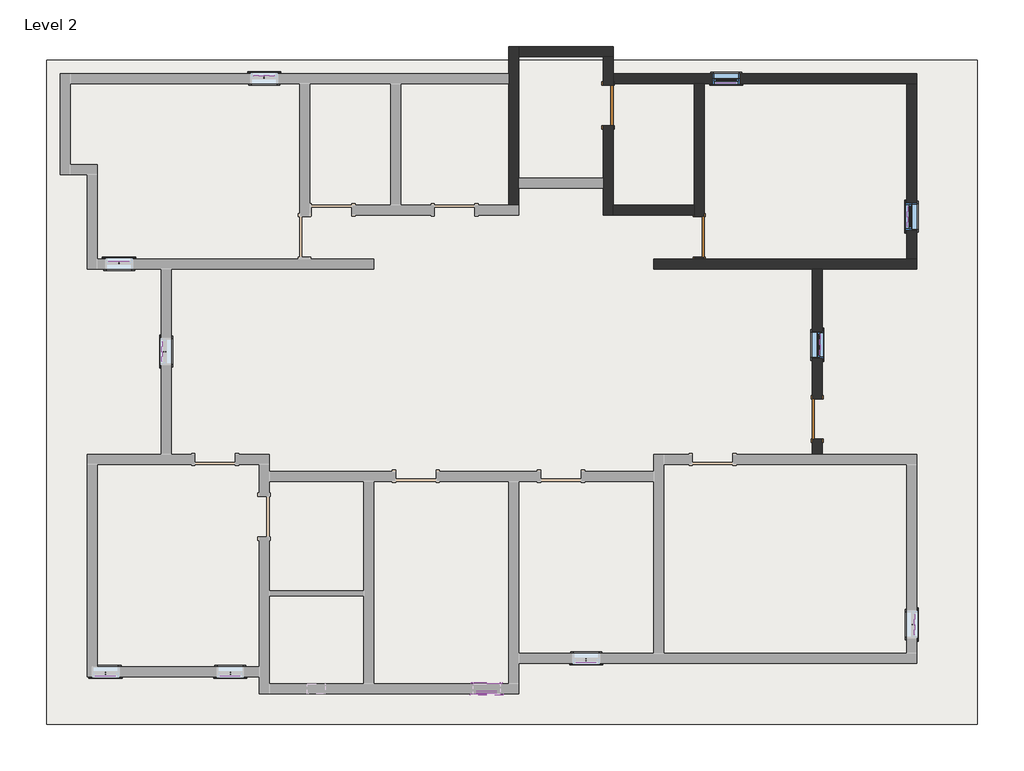
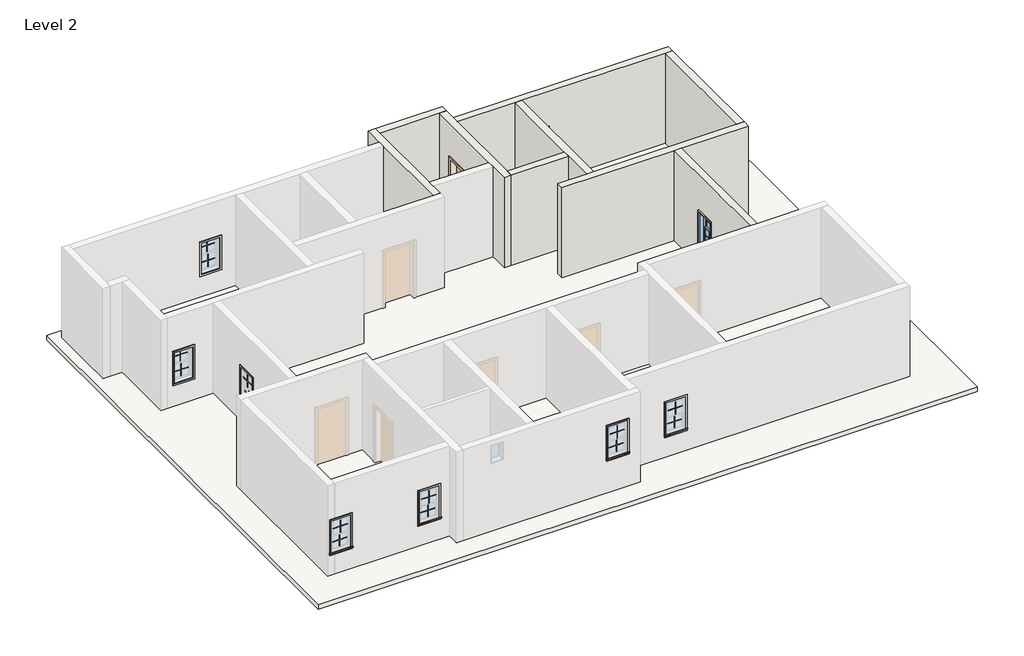
# One storey, part 2 of 2: 44 proxies, 9 walls, 3 doors, 3 windows, 1 roof.
"""IFC4 building model written with IfcOpenShell, lengths in millimetres."""

from ifc_helpers import new_model, si_unit, frame, origin, place, context, project, spatial, polyline, outline, extrude, faceted_brep, transform, mapped, element, save
from components import muntin_pattern_2x2_muntin_pattern_2x2_eba6c5fb, trim_window_exterior_flat_with_sill_278e6a94, trim_window_interior_flat_picture_frame_e9fd5f45, door_89fc3733, door_ef0d591a, window_d92165b9

model = new_model("IFC4")

# Units and contexts
model_context = context("Model", 3, world=origin())
ifc_project = project(units=[si_unit("LENGTHUNIT", "METRE", prefix="MILLI")], contexts=[model_context])

# Site, building, storey
site = spatial("IfcSite", under=ifc_project)
building = spatial("IfcBuilding", under=site)
storey = spatial("IfcBuildingStorey", under=building, Name="Level 2", Elevation=3200.4)

# Proxies
placement = place(None, origin())
muntin_pattern_2x2_muntin_pattern_2x2_shape = muntin_pattern_2x2_muntin_pattern_2x2_eba6c5fb(model_context)
element("IfcBuildingElementProxy", 1, Name="Muntin Pattern_2x2 : Muntin Pattern_2x2", ObjectType="Muntin Pattern_2x2 : Muntin Pattern_2x2", at=placement, inside=storey, context=model_context, shape_type="MappedRepresentation", body=[
    mapped(muntin_pattern_2x2_muntin_pattern_2x2_shape, transform((-9484.8415084, 7932.7685985, 4670.425), x_axis=(1.0, 0.0, 0.0), y_axis=(0.0, 1.0, 0.0), z_axis=(0.0, 0.0, 1.0))),
])
element("IfcBuildingElementProxy", 2, Name="Muntin Pattern_2x2 : Muntin Pattern_2x2", ObjectType="Muntin Pattern_2x2 : Muntin Pattern_2x2", at=placement, inside=storey, context=model_context, shape_type="MappedRepresentation", body=[
    mapped(muntin_pattern_2x2_muntin_pattern_2x2_shape, transform((-9484.8415084, 7888.3185985, 4191.0), x_axis=(1.0, 0.0, 0.0), y_axis=(0.0, 1.0, 0.0), z_axis=(0.0, 0.0, 1.0))),
])
element("IfcBuildingElementProxy", 3, Name="Muntin Pattern_2x2 : Muntin Pattern_2x2", ObjectType="Muntin Pattern_2x2 : Muntin Pattern_2x2", at=placement, inside=storey, context=model_context, shape_type="MappedRepresentation", body=[
    mapped(muntin_pattern_2x2_muntin_pattern_2x2_shape, transform((-12761.4415084, 3741.7685985, 4670.425), x_axis=(1.0, 0.0, 0.0), y_axis=(0.0, 1.0, 0.0), z_axis=(0.0, 0.0, 1.0))),
])
element("IfcBuildingElementProxy", 4, Name="Muntin Pattern_2x2 : Muntin Pattern_2x2", ObjectType="Muntin Pattern_2x2 : Muntin Pattern_2x2", at=placement, inside=storey, context=model_context, shape_type="MappedRepresentation", body=[
    mapped(muntin_pattern_2x2_muntin_pattern_2x2_shape, transform((-12761.4415084, 3697.3185985, 4191.0), x_axis=(1.0, 0.0, 0.0), y_axis=(0.0, 1.0, 0.0), z_axis=(0.0, 0.0, 1.0))),
])
element("IfcBuildingElementProxy", 5, Name="Muntin Pattern_2x2 : Muntin Pattern_2x2", ObjectType="Muntin Pattern_2x2 : Muntin Pattern_2x2", at=placement, inside=storey, context=model_context, shape_type="MappedRepresentation", body=[
    mapped(muntin_pattern_2x2_muntin_pattern_2x2_shape, transform((-13066.2415084, -5637.1814015, 4670.425), x_axis=(-1.0, 0.0, 0.0), y_axis=(0.0, -1.0, 0.0), z_axis=(0.0, 0.0, 1.0))),
])
element("IfcBuildingElementProxy", 6, Name="Muntin Pattern_2x2 : Muntin Pattern_2x2", ObjectType="Muntin Pattern_2x2 : Muntin Pattern_2x2", at=placement, inside=storey, context=model_context, shape_type="MappedRepresentation", body=[
    mapped(muntin_pattern_2x2_muntin_pattern_2x2_shape, transform((-13066.2415084, -5592.7314015, 4191.0), x_axis=(-1.0, 0.0, 0.0), y_axis=(0.0, -1.0, 0.0), z_axis=(0.0, 0.0, 1.0))),
])
element("IfcBuildingElementProxy", 7, Name="Muntin Pattern_2x2 : Muntin Pattern_2x2", ObjectType="Muntin Pattern_2x2 : Muntin Pattern_2x2", at=placement, inside=storey, context=model_context, shape_type="MappedRepresentation", body=[
    mapped(muntin_pattern_2x2_muntin_pattern_2x2_shape, transform((-10246.8415084, -5637.1814015, 4670.425), x_axis=(-1.0, 0.0, 0.0), y_axis=(0.0, -1.0, 0.0), z_axis=(0.0, 0.0, 1.0))),
])
element("IfcBuildingElementProxy", 8, Name="Muntin Pattern_2x2 : Muntin Pattern_2x2", ObjectType="Muntin Pattern_2x2 : Muntin Pattern_2x2", at=placement, inside=storey, context=model_context, shape_type="MappedRepresentation", body=[
    mapped(muntin_pattern_2x2_muntin_pattern_2x2_shape, transform((-10246.8415084, -5592.7314015, 4191.0), x_axis=(-1.0, 0.0, 0.0), y_axis=(0.0, -1.0, 0.0), z_axis=(0.0, 0.0, 1.0))),
])
element("IfcBuildingElementProxy", 9, Name="Muntin Pattern_2x2 : Muntin Pattern_2x2", ObjectType="Muntin Pattern_2x2 : Muntin Pattern_2x2", at=placement, inside=storey, context=model_context, shape_type="MappedRepresentation", body=[
    mapped(muntin_pattern_2x2_muntin_pattern_2x2_shape, transform((954.5584916, 7774.0185985, 4670.425), x_axis=(-1.0, 0.0, 0.0), y_axis=(0.0, -1.0, 0.0), z_axis=(0.0, 0.0, 1.0))),
])
element("IfcBuildingElementProxy", 10, Name="Muntin Pattern_2x2 : Muntin Pattern_2x2", ObjectType="Muntin Pattern_2x2 : Muntin Pattern_2x2", at=placement, inside=storey, context=model_context, shape_type="MappedRepresentation", body=[
    mapped(muntin_pattern_2x2_muntin_pattern_2x2_shape, transform((954.5584916, 7818.4685985, 4191.0), x_axis=(-1.0, 0.0, 0.0), y_axis=(0.0, -1.0, 0.0), z_axis=(0.0, 0.0, 1.0))),
])
element("IfcBuildingElementProxy", 11, Name="Muntin Pattern_2x2 : Muntin Pattern_2x2", ObjectType="Muntin Pattern_2x2 : Muntin Pattern_2x2", at=placement, inside=storey, context=model_context, shape_type="MappedRepresentation", body=[
    mapped(muntin_pattern_2x2_muntin_pattern_2x2_shape, transform((-11774.0165084, 1681.1935985, 4670.425), x_axis=(0.0, 1.0, 0.0), y_axis=(-1.0, 0.0, 0.0), z_axis=(0.0, 0.0, 1.0))),
])
element("IfcBuildingElementProxy", 12, Name="Muntin Pattern_2x2 : Muntin Pattern_2x2", ObjectType="Muntin Pattern_2x2 : Muntin Pattern_2x2", at=placement, inside=storey, context=model_context, shape_type="MappedRepresentation", body=[
    mapped(muntin_pattern_2x2_muntin_pattern_2x2_shape, transform((-11729.5665084, 1681.1935985, 4191.0), x_axis=(0.0, 1.0, 0.0), y_axis=(-1.0, 0.0, 0.0), z_axis=(0.0, 0.0, 1.0))),
])
element("IfcBuildingElementProxy", 13, Name="Muntin Pattern_2x2 : Muntin Pattern_2x2", ObjectType="Muntin Pattern_2x2 : Muntin Pattern_2x2", at=placement, inside=storey, context=model_context, shape_type="MappedRepresentation", body=[
    mapped(muntin_pattern_2x2_muntin_pattern_2x2_shape, transform((-2207.7415084, -5332.3814015, 4670.425), x_axis=(-1.0, 0.0, 0.0), y_axis=(0.0, -1.0, 0.0), z_axis=(0.0, 0.0, 1.0))),
])
element("IfcBuildingElementProxy", 14, Name="Muntin Pattern_2x2 : Muntin Pattern_2x2", ObjectType="Muntin Pattern_2x2 : Muntin Pattern_2x2", at=placement, inside=storey, context=model_context, shape_type="MappedRepresentation", body=[
    mapped(muntin_pattern_2x2_muntin_pattern_2x2_shape, transform((-2207.7415084, -5287.9314015, 4191.0), x_axis=(-1.0, 0.0, 0.0), y_axis=(0.0, -1.0, 0.0), z_axis=(0.0, 0.0, 1.0))),
])
element("IfcBuildingElementProxy", 15, Name="Muntin Pattern_2x2 : Muntin Pattern_2x2", ObjectType="Muntin Pattern_2x2 : Muntin Pattern_2x2", at=placement, inside=storey, context=model_context, shape_type="MappedRepresentation", body=[
    mapped(muntin_pattern_2x2_muntin_pattern_2x2_shape, transform((5224.9334916, -4491.0064015, 4670.425), x_axis=(0.0, -1.0, 0.0), y_axis=(1.0, 0.0, 0.0), z_axis=(0.0, 0.0, 1.0))),
])
element("IfcBuildingElementProxy", 16, Name="Muntin Pattern_2x2 : Muntin Pattern_2x2", ObjectType="Muntin Pattern_2x2 : Muntin Pattern_2x2", at=placement, inside=storey, context=model_context, shape_type="MappedRepresentation", body=[
    mapped(muntin_pattern_2x2_muntin_pattern_2x2_shape, transform((5180.4834916, -4491.0064015, 4191.0), x_axis=(0.0, -1.0, 0.0), y_axis=(1.0, 0.0, 0.0), z_axis=(0.0, 0.0, 1.0))),
])
element("IfcBuildingElementProxy", 17, Name="Muntin Pattern_2x2 : Muntin Pattern_2x2", ObjectType="Muntin Pattern_2x2 : Muntin Pattern_2x2", at=placement, inside=storey, context=model_context, shape_type="MappedRepresentation", body=[
    mapped(muntin_pattern_2x2_muntin_pattern_2x2_shape, transform((3091.3334916, 1833.5935985, 4670.425), x_axis=(0.0, -1.0, 0.0), y_axis=(1.0, 0.0, 0.0), z_axis=(0.0, 0.0, 1.0))),
])
element("IfcBuildingElementProxy", 18, Name="Muntin Pattern_2x2 : Muntin Pattern_2x2", ObjectType="Muntin Pattern_2x2 : Muntin Pattern_2x2", at=placement, inside=storey, context=model_context, shape_type="MappedRepresentation", body=[
    mapped(muntin_pattern_2x2_muntin_pattern_2x2_shape, transform((3046.8834916, 1833.5935985, 4191.0), x_axis=(0.0, -1.0, 0.0), y_axis=(1.0, 0.0, 0.0), z_axis=(0.0, 0.0, 1.0))),
])
element("IfcBuildingElementProxy", 19, Name="Muntin Pattern_2x2 : Muntin Pattern_2x2", ObjectType="Muntin Pattern_2x2 : Muntin Pattern_2x2", at=placement, inside=storey, context=model_context, shape_type="MappedRepresentation", body=[
    mapped(muntin_pattern_2x2_muntin_pattern_2x2_shape, transform((5066.1834916, 4729.1935985, 4670.425), x_axis=(0.0, 1.0, 0.0), y_axis=(-1.0, 0.0, 0.0), z_axis=(0.0, 0.0, 1.0))),
])
element("IfcBuildingElementProxy", 20, Name="Muntin Pattern_2x2 : Muntin Pattern_2x2", ObjectType="Muntin Pattern_2x2 : Muntin Pattern_2x2", at=placement, inside=storey, context=model_context, shape_type="MappedRepresentation", body=[
    mapped(muntin_pattern_2x2_muntin_pattern_2x2_shape, transform((5110.6334916, 4729.1935985, 4191.0), x_axis=(0.0, 1.0, 0.0), y_axis=(-1.0, 0.0, 0.0), z_axis=(0.0, 0.0, 1.0))),
])
element("IfcBuildingElementProxy", 21, Name="Muntin Pattern_2x2 : Muntin Pattern_2x2", ObjectType="Muntin Pattern_2x2 : Muntin Pattern_2x2", at=placement, inside=storey, context=model_context, shape_type="MappedRepresentation", body=[
    mapped(muntin_pattern_2x2_muntin_pattern_2x2_shape, transform((-4455.6415084, -6018.2598078, 5074.2137433), x_axis=(-1.0, 0.0, 0.0), y_axis=(0.0, -1.0, 0.0), z_axis=(0.0, 0.0, 1.0))),
])
element("IfcBuildingElementProxy", 22, Name="Muntin Pattern_2x2 : Muntin Pattern_2x2", ObjectType="Muntin Pattern_2x2 : Muntin Pattern_2x2", at=placement, inside=storey, context=model_context, shape_type="MappedRepresentation", body=[
    mapped(muntin_pattern_2x2_muntin_pattern_2x2_shape, transform((-4455.6415084, -5973.8098078, 4594.7887433), x_axis=(-1.0, 0.0, 0.0), y_axis=(0.0, -1.0, 0.0), z_axis=(0.0, 0.0, 1.0))),
])
trim_window_exterior_flat_with_sill_shape = trim_window_exterior_flat_with_sill_278e6a94(model_context)
element("IfcBuildingElementProxy", 23, Name="Trim-Window-Exterior-Flat : with Sill", ObjectType="Trim-Window-Exterior-Flat : with Sill", at=placement, inside=storey, context=model_context, shape_type="MappedRepresentation", body=[
    mapped(trim_window_exterior_flat_with_sill_shape, transform((-9484.8415084, 7967.6935985, 5181.6), x_axis=(-1.0, 0.0, 0.0), y_axis=(0.0, 0.0, 1.0), z_axis=(0.0, 1.0, 0.0))),
])
element("IfcBuildingElementProxy", 24, Name="Trim-Window-Exterior-Flat : with Sill", ObjectType="Trim-Window-Exterior-Flat : with Sill", at=placement, inside=storey, context=model_context, shape_type="MappedRepresentation", body=[
    mapped(trim_window_exterior_flat_with_sill_shape, transform((-12761.4415084, 3776.6935985, 5181.6), x_axis=(-1.0, 0.0, 0.0), y_axis=(0.0, 0.0, 1.0), z_axis=(0.0, 1.0, 0.0))),
])
element("IfcBuildingElementProxy", 25, Name="Trim-Window-Exterior-Flat : with Sill", ObjectType="Trim-Window-Exterior-Flat : with Sill", at=placement, inside=storey, context=model_context, shape_type="MappedRepresentation", body=[
    mapped(trim_window_exterior_flat_with_sill_shape, transform((-13066.2415084, -5672.1064015, 5181.6), x_axis=(1.0, 0.0, 0.0), y_axis=(0.0, 0.0, 1.0), z_axis=(0.0, -1.0, 0.0))),
])
element("IfcBuildingElementProxy", 26, Name="Trim-Window-Exterior-Flat : with Sill", ObjectType="Trim-Window-Exterior-Flat : with Sill", at=placement, inside=storey, context=model_context, shape_type="MappedRepresentation", body=[
    mapped(trim_window_exterior_flat_with_sill_shape, transform((-10246.8415084, -5672.1064015, 5181.6), x_axis=(1.0, 0.0, 0.0), y_axis=(0.0, 0.0, 1.0), z_axis=(0.0, -1.0, 0.0))),
])
element("IfcBuildingElementProxy", 27, Name="Trim-Window-Exterior-Flat : with Sill", ObjectType="Trim-Window-Exterior-Flat : with Sill", at=placement, inside=storey, context=model_context, shape_type="MappedRepresentation", body=[
    mapped(trim_window_exterior_flat_with_sill_shape, transform((954.5584916, 7739.0935985, 5181.6), x_axis=(1.0, 0.0, 0.0), y_axis=(0.0, 0.0, 1.0), z_axis=(0.0, -1.0, 0.0))),
])
element("IfcBuildingElementProxy", 28, Name="Trim-Window-Exterior-Flat : with Sill", ObjectType="Trim-Window-Exterior-Flat : with Sill", at=placement, inside=storey, context=model_context, shape_type="MappedRepresentation", body=[
    mapped(trim_window_exterior_flat_with_sill_shape, transform((-11808.9415084, 1681.1935985, 5181.6), x_axis=(0.0, -1.0, 0.0), y_axis=(0.0, 0.0, 1.0), z_axis=(-1.0, 0.0, 0.0))),
])
element("IfcBuildingElementProxy", 29, Name="Trim-Window-Exterior-Flat : with Sill", ObjectType="Trim-Window-Exterior-Flat : with Sill", at=placement, inside=storey, context=model_context, shape_type="MappedRepresentation", body=[
    mapped(trim_window_exterior_flat_with_sill_shape, transform((-2207.7415084, -5367.3064015, 5181.6), x_axis=(1.0, 0.0, 0.0), y_axis=(0.0, 0.0, 1.0), z_axis=(0.0, -1.0, 0.0))),
])
element("IfcBuildingElementProxy", 30, Name="Trim-Window-Exterior-Flat : with Sill", ObjectType="Trim-Window-Exterior-Flat : with Sill", at=placement, inside=storey, context=model_context, shape_type="MappedRepresentation", body=[
    mapped(trim_window_exterior_flat_with_sill_shape, transform((5259.8584916, -4491.0064015, 5181.6), x_axis=(0.0, 1.0, 0.0), y_axis=(0.0, 0.0, 1.0), z_axis=(1.0, 0.0, 0.0))),
])
element("IfcBuildingElementProxy", 31, Name="Trim-Window-Exterior-Flat : with Sill", ObjectType="Trim-Window-Exterior-Flat : with Sill", at=placement, inside=storey, context=model_context, shape_type="MappedRepresentation", body=[
    mapped(trim_window_exterior_flat_with_sill_shape, transform((3126.2584916, 1833.5935985, 5181.6), x_axis=(0.0, 1.0, 0.0), y_axis=(0.0, 0.0, 1.0), z_axis=(1.0, 0.0, 0.0))),
])
element("IfcBuildingElementProxy", 32, Name="Trim-Window-Exterior-Flat : with Sill", ObjectType="Trim-Window-Exterior-Flat : with Sill", at=placement, inside=storey, context=model_context, shape_type="MappedRepresentation", body=[
    mapped(trim_window_exterior_flat_with_sill_shape, transform((5031.2584916, 4729.1935985, 5181.6), x_axis=(0.0, -1.0, 0.0), y_axis=(0.0, 0.0, 1.0), z_axis=(-1.0, 0.0, 0.0))),
])
element("IfcBuildingElementProxy", 33, Name="Trim-Window-Exterior-Flat : with Sill", ObjectType="Trim-Window-Exterior-Flat : with Sill", at=placement, inside=storey, context=model_context, shape_type="MappedRepresentation", body=[
    mapped(trim_window_exterior_flat_with_sill_shape, transform((-4455.6415084, -6053.1848078, 5585.3887433), x_axis=(1.0, 0.0, 0.0), y_axis=(0.0, 0.0, 1.0), z_axis=(0.0, -1.0, 0.0))),
])
trim_window_interior_flat_picture_frame_shape = trim_window_interior_flat_picture_frame_e9fd5f45(model_context)
element("IfcBuildingElementProxy", 34, Name="Trim-Window-Interior-Flat : Picture Frame", ObjectType="Trim-Window-Interior-Flat : Picture Frame", at=placement, inside=storey, context=model_context, shape_type="MappedRepresentation", body=[
    mapped(trim_window_interior_flat_picture_frame_shape, transform((-9484.8415084, 7739.0935985, 5181.6), x_axis=(1.0, 0.0, 0.0), y_axis=(0.0, 0.0, 1.0), z_axis=(0.0, -1.0, 0.0))),
])
element("IfcBuildingElementProxy", 35, Name="Trim-Window-Interior-Flat : Picture Frame", ObjectType="Trim-Window-Interior-Flat : Picture Frame", at=placement, inside=storey, context=model_context, shape_type="MappedRepresentation", body=[
    mapped(trim_window_interior_flat_picture_frame_shape, transform((-12761.4415084, 3548.0935985, 5181.6), x_axis=(1.0, 0.0, 0.0), y_axis=(0.0, 0.0, 1.0), z_axis=(0.0, -1.0, 0.0))),
])
element("IfcBuildingElementProxy", 36, Name="Trim-Window-Interior-Flat : Picture Frame", ObjectType="Trim-Window-Interior-Flat : Picture Frame", at=placement, inside=storey, context=model_context, shape_type="MappedRepresentation", body=[
    mapped(trim_window_interior_flat_picture_frame_shape, transform((-13066.2415084, -5443.5064015, 5181.6), x_axis=(-1.0, 0.0, 0.0), y_axis=(0.0, 0.0, 1.0), z_axis=(0.0, 1.0, 0.0))),
])
element("IfcBuildingElementProxy", 37, Name="Trim-Window-Interior-Flat : Picture Frame", ObjectType="Trim-Window-Interior-Flat : Picture Frame", at=placement, inside=storey, context=model_context, shape_type="MappedRepresentation", body=[
    mapped(trim_window_interior_flat_picture_frame_shape, transform((-10246.8415084, -5443.5064015, 5181.6), x_axis=(-1.0, 0.0, 0.0), y_axis=(0.0, 0.0, 1.0), z_axis=(0.0, 1.0, 0.0))),
])
element("IfcBuildingElementProxy", 38, Name="Trim-Window-Interior-Flat : Picture Frame", ObjectType="Trim-Window-Interior-Flat : Picture Frame", at=placement, inside=storey, context=model_context, shape_type="MappedRepresentation", body=[
    mapped(trim_window_interior_flat_picture_frame_shape, transform((954.5584916, 7967.6935985, 5181.6), x_axis=(-1.0, 0.0, 0.0), y_axis=(0.0, 0.0, 1.0), z_axis=(0.0, 1.0, 0.0))),
])
element("IfcBuildingElementProxy", 39, Name="Trim-Window-Interior-Flat : Picture Frame", ObjectType="Trim-Window-Interior-Flat : Picture Frame", at=placement, inside=storey, context=model_context, shape_type="MappedRepresentation", body=[
    mapped(trim_window_interior_flat_picture_frame_shape, transform((-11580.3415084, 1681.1935985, 5181.6), x_axis=(0.0, 1.0, 0.0), y_axis=(0.0, 0.0, 1.0), z_axis=(1.0, 0.0, 0.0))),
])
element("IfcBuildingElementProxy", 40, Name="Trim-Window-Interior-Flat : Picture Frame", ObjectType="Trim-Window-Interior-Flat : Picture Frame", at=placement, inside=storey, context=model_context, shape_type="MappedRepresentation", body=[
    mapped(trim_window_interior_flat_picture_frame_shape, transform((-2207.7415084, -5138.7064015, 5181.6), x_axis=(-1.0, 0.0, 0.0), y_axis=(0.0, 0.0, 1.0), z_axis=(0.0, 1.0, 0.0))),
])
element("IfcBuildingElementProxy", 41, Name="Trim-Window-Interior-Flat : Picture Frame", ObjectType="Trim-Window-Interior-Flat : Picture Frame", at=placement, inside=storey, context=model_context, shape_type="MappedRepresentation", body=[
    mapped(trim_window_interior_flat_picture_frame_shape, transform((5031.2584916, -4491.0064015, 5181.6), x_axis=(0.0, -1.0, 0.0), y_axis=(0.0, 0.0, 1.0), z_axis=(-1.0, 0.0, 0.0))),
])
element("IfcBuildingElementProxy", 42, Name="Trim-Window-Interior-Flat : Picture Frame", ObjectType="Trim-Window-Interior-Flat : Picture Frame", at=placement, inside=storey, context=model_context, shape_type="MappedRepresentation", body=[
    mapped(trim_window_interior_flat_picture_frame_shape, transform((2897.6584916, 1833.5935985, 5181.6), x_axis=(0.0, -1.0, 0.0), y_axis=(0.0, 0.0, 1.0), z_axis=(-1.0, 0.0, 0.0))),
])
element("IfcBuildingElementProxy", 43, Name="Trim-Window-Interior-Flat : Picture Frame", ObjectType="Trim-Window-Interior-Flat : Picture Frame", at=placement, inside=storey, context=model_context, shape_type="MappedRepresentation", body=[
    mapped(trim_window_interior_flat_picture_frame_shape, transform((5259.8584916, 4729.1935985, 5181.6), x_axis=(0.0, 1.0, 0.0), y_axis=(0.0, 0.0, 1.0), z_axis=(1.0, 0.0, 0.0))),
])
element("IfcBuildingElementProxy", 44, Name="Trim-Window-Interior-Flat : Picture Frame", ObjectType="Trim-Window-Interior-Flat : Picture Frame", at=placement, inside=storey, context=model_context, shape_type="MappedRepresentation", body=[
    mapped(trim_window_interior_flat_picture_frame_shape, transform((-4455.6415084, -5824.5848078, 5585.3887433), x_axis=(-1.0, 0.0, 0.0), y_axis=(0.0, 0.0, 1.0), z_axis=(0.0, 1.0, 0.0))),
])

# Doors
door_shape = door_89fc3733(model_context)
element("IfcDoor", 45, ObjectType="Single-Flush : 36\" x 80\"", at=placement, inside=storey, context=model_context, shape_type="MappedRepresentation", body=[
    mapped(door_shape, transform((344.9584916, 4271.9935985, 3200.4), x_axis=(0.0, -1.0, 0.0), y_axis=(1.0, 0.0, 0.0), z_axis=(0.0, 0.0, 1.0))),
])
door_2_shape = door_ef0d591a(model_context)
element("IfcDoor", 46, ObjectType="Single-Flush : 36\" x 80\"", at=placement, inside=storey, context=model_context, shape_type="MappedRepresentation", body=[
    mapped(door_2_shape, transform((-1712.4415084, 7243.7935985, 3200.4), x_axis=(0.0, 1.0, 0.0), y_axis=(-1.0, 0.0, 0.0), z_axis=(0.0, 0.0, 1.0))),
])
element("IfcDoor", 47, ObjectType="Single-Flush : 36\" x 80\"", at=placement, inside=storey, context=model_context, shape_type="MappedRepresentation", body=[
    mapped(door_2_shape, transform((3011.9584916, 157.1935985, 3200.4), x_axis=(0.0, -1.0, 0.0), y_axis=(1.0, 0.0, 0.0), z_axis=(0.0, 0.0, 1.0))),
])

# Roof
element("IfcRoof", 48, ObjectType="6\"", at=placement, inside=storey, context=model_context, shape_type="SweptSolid", body=[
    extrude(outline(polyline([(-14399.7415084, 8272.4935985), (6631.4584916, 8272.4935985), (6631.4584916, -6739.2866284), (-14399.7415084, -6739.2866284), (-14399.7415084, 8272.4935985)])), frame((0.0, 0.0, 3200.4), z_axis=(0.0, 0.0, 1.0), x_axis=(1.0, 0.0, 0.0)), (0.0, 0.0, 1.0), 152.4),
])

# Walls
element("IfcWall", 49, ObjectType="9\"", at=placement, inside=storey, context=model_context, shape_type="Brep", body=[
    faceted_brep([(-3960.3415084, 8577.2935985, 3200.4), (-3960.3415084, 7967.6935985, 3200.4), (-3960.3415084, 7739.0935985, 3200.4), (-3960.3415084, 4995.8935985, 3200.4), (-3960.3415084, 4995.8935985, 6400.8), (-3960.3415084, 7739.0935985, 6400.8), (-3960.3415084, 7967.6935985, 6400.8), (-3960.3415084, 8577.2935985, 6400.8), (-3731.7415084, 8577.2935985, 3200.4), (-3731.7415084, 8577.2935985, 6400.8), (-3731.7415084, 8348.6935985, 6400.8), (-3731.7415084, 5605.4935985, 6400.8), (-3731.7415084, 5376.8935985, 6400.8), (-3731.7415084, 4995.8935985, 6400.8), (-3731.7415084, 4995.8935985, 3200.4), (-3731.7415084, 5376.8935985, 3200.4), (-3731.7415084, 5605.4935985, 3200.4), (-3731.7415084, 8348.6935985, 3200.4)], [[[0, 1, 2, 3, 4, 5, 6, 7]], [[8, 9, 10, 11, 12, 13, 14, 15, 16, 17]], [[3, 2, 1, 0, 8, 17, 16, 15, 14]], [[7, 6, 5, 4, 13, 12, 11, 10, 9]], [[4, 3, 14, 13]], [[0, 7, 9, 8]]]),
])
element("IfcWall", 50, ObjectType="9\"", at=placement, inside=storey, context=model_context, shape_type="Brep", body=[
    faceted_brep([(-1598.1415084, 8577.2935985, 3200.4), (-3731.7415084, 8577.2935985, 3200.4), (-3731.7415084, 8577.2935985, 6400.8), (-1598.1415084, 8577.2935985, 6400.8), (-1598.1415084, 8348.6935985, 3200.4), (-1598.1415084, 8348.6935985, 6400.8), (-1826.7415084, 8348.6935985, 6400.8), (-3731.7415084, 8348.6935985, 6400.8), (-3731.7415084, 8348.6935985, 3200.4), (-1826.7415084, 8348.6935985, 3200.4)], [[[0, 1, 2, 3]], [[4, 5, 6, 7, 8, 9]], [[1, 0, 4, 9, 8]], [[3, 2, 7, 6, 5]], [[2, 1, 8, 7]], [[0, 3, 5, 4]]]),
])
element("IfcWall", 51, ObjectType="9\"", at=placement, inside=storey, context=model_context, shape_type="Brep", body=[
    faceted_brep([(-1598.1415084, 7700.9935985, 5232.4), (-1598.1415084, 7700.9935985, 3200.4), (-1598.1415084, 7739.0935985, 3200.4), (-1598.1415084, 7967.6935985, 3200.4), (-1598.1415084, 8348.6935985, 3200.4), (-1598.1415084, 8348.6935985, 6400.8), (-1598.1415084, 7967.6935985, 6400.8), (-1598.1415084, 7739.0935985, 6400.8), (-1598.1415084, 4995.8935985, 6400.8), (-1598.1415084, 4767.2935985, 6400.8), (-1598.1415084, 4767.2935985, 3200.4), (-1598.1415084, 4995.8935985, 3200.4), (-1598.1415084, 6786.5935985, 3200.4), (-1598.1415084, 6786.5935985, 5232.4), (-1826.7415084, 8348.6935985, 3200.4), (-1826.7415084, 7700.9935985, 3200.4), (-1826.7415084, 7700.9935985, 5232.4), (-1826.7415084, 6786.5935985, 5232.4), (-1826.7415084, 6786.5935985, 3200.4), (-1826.7415084, 5605.4935985, 3200.4), (-1826.7415084, 5376.8935985, 3200.4), (-1826.7415084, 4767.2935985, 3200.4), (-1826.7415084, 4767.2935985, 6400.8), (-1826.7415084, 5376.8935985, 6400.8), (-1826.7415084, 5605.4935985, 6400.8), (-1826.7415084, 8348.6935985, 6400.8)], [[[0, 1, 2, 3, 4, 5, 6, 7, 8, 9, 10, 11, 12, 13]], [[14, 15, 16, 17, 18, 19, 20, 21, 22, 23, 24, 25]], [[12, 11, 10, 21, 20, 19, 18]], [[4, 3, 2, 1, 15, 14]], [[9, 8, 7, 6, 5, 25, 24, 23, 22]], [[5, 4, 14, 25]], [[10, 9, 22, 21]], [[16, 15, 1, 0]], [[17, 16, 0, 13]], [[18, 17, 13, 12]]]),
])
element("IfcWall", 52, ObjectType="9\"", at=placement, inside=storey, context=model_context, shape_type="SweptSolid", body=[
    extrude(outline(polyline([(-1598.1415084, 4995.8935985), (230.6584916, 4995.8935985), (230.6584916, 4767.2935985), (-1598.1415084, 4767.2935985), (-1598.1415084, 4995.8935985)])), frame((0.0, 0.0, 3200.4), z_axis=(0.0, 0.0, 1.0), x_axis=(1.0, 0.0, 0.0)), (0.0, 0.0, 1.0), 3200.4),
])
element("IfcWall", 53, ObjectType="9\"", at=placement, inside=storey, context=model_context, shape_type="Brep", body=[
    faceted_brep([(-683.7415084, 3548.0935985, 3200.4), (2897.6584916, 3548.0935985, 3200.4), (3126.2584916, 3548.0935985, 3200.4), (5259.8584916, 3548.0935985, 3200.4), (5259.8584916, 3548.0935985, 6400.8), (3126.2584916, 3548.0935985, 6400.8), (2897.6584916, 3548.0935985, 6400.8), (-683.7415084, 3548.0935985, 6400.8), (-683.7415084, 3776.6935985, 3200.4), (-683.7415084, 3776.6935985, 6400.8), (230.6584916, 3776.6935985, 6400.8), (459.2584916, 3776.6935985, 6400.8), (5031.2584916, 3776.6935985, 6400.8), (5259.8584916, 3776.6935985, 6400.8), (5259.8584916, 3776.6935985, 3200.4), (5031.2584916, 3776.6935985, 3200.4), (459.2584916, 3776.6935985, 3200.4), (230.6584916, 3776.6935985, 3200.4)], [[[0, 1, 2, 3, 4, 5, 6, 7]], [[8, 9, 10, 11, 12, 13, 14, 15, 16, 17]], [[3, 2, 1, 0, 8, 17, 16, 15, 14]], [[7, 6, 5, 4, 13, 12, 11, 10, 9]], [[0, 7, 9, 8]], [[4, 3, 14, 13]]]),
])
element("IfcWall", 54, ObjectType="9\"", at=placement, inside=storey, context=model_context, shape_type="Brep", body=[
    faceted_brep([(230.6584916, 3814.7935985, 5232.4), (230.6584916, 3814.7935985, 3200.4), (230.6584916, 3776.6935985, 3200.4), (230.6584916, 3776.6935985, 6400.8), (230.6584916, 4767.2935985, 6400.8), (230.6584916, 4995.8935985, 6400.8), (230.6584916, 7739.0935985, 6400.8), (230.6584916, 7739.0935985, 3200.4), (230.6584916, 4995.8935985, 3200.4), (230.6584916, 4767.2935985, 3200.4), (230.6584916, 4729.1935985, 3200.4), (230.6584916, 4729.1935985, 5232.4), (459.2584916, 3776.6935985, 3200.4), (459.2584916, 3814.7935985, 3200.4), (459.2584916, 3814.7935985, 5232.4), (459.2584916, 4729.1935985, 5232.4), (459.2584916, 4729.1935985, 3200.4), (459.2584916, 7739.0935985, 3200.4), (459.2584916, 7739.0935985, 6400.8), (459.2584916, 3776.6935985, 6400.8)], [[[0, 1, 2, 3, 4, 5, 6, 7, 8, 9, 10, 11]], [[12, 13, 14, 15, 16, 17, 18, 19]], [[2, 1, 13, 12]], [[10, 9, 8, 7, 17, 16]], [[6, 5, 4, 3, 19, 18]], [[3, 2, 12, 19]], [[7, 6, 18, 17]], [[14, 13, 1, 0]], [[15, 14, 0, 11]], [[16, 15, 11, 10]]]),
])
element("IfcWall", 55, ObjectType="9\"", at=placement, inside=storey, context=model_context, shape_type="Brep", body=[
    faceted_brep([(5259.8584916, 7967.6935985, 3200.4), (-1598.1415084, 7967.6935985, 3200.4), (-1598.1415084, 7967.6935985, 6400.8), (5259.8584916, 7967.6935985, 6400.8), (1259.3584916, 7967.6935985, 5181.6), (649.7584916, 7967.6935985, 5181.6), (649.7584916, 7967.6935985, 4114.8), (1259.3584916, 7967.6935985, 4114.8), (5259.8584916, 7739.0935985, 3200.4), (5259.8584916, 7739.0935985, 6400.8), (5031.2584916, 7739.0935985, 6400.8), (459.2584916, 7739.0935985, 6400.8), (230.6584916, 7739.0935985, 6400.8), (-1598.1415084, 7739.0935985, 6400.8), (-1598.1415084, 7739.0935985, 3200.4), (230.6584916, 7739.0935985, 3200.4), (459.2584916, 7739.0935985, 3200.4), (5031.2584916, 7739.0935985, 3200.4), (1259.3584916, 7739.0935985, 5181.6), (1259.3584916, 7739.0935985, 4114.8), (649.7584916, 7739.0935985, 4114.8), (649.7584916, 7739.0935985, 5181.6)], [[[0, 1, 2, 3], [4, 5, 6, 7]], [[8, 9, 10, 11, 12, 13, 14, 15, 16, 17], [18, 19, 20, 21]], [[1, 0, 8, 17, 16, 15, 14]], [[3, 2, 13, 12, 11, 10, 9]], [[2, 1, 14, 13]], [[0, 3, 9, 8]], [[19, 18, 4, 7]], [[20, 19, 7, 6]], [[21, 20, 6, 5]], [[18, 21, 5, 4]]]),
])
element("IfcWall", 56, ObjectType="9\"", at=placement, inside=storey, context=model_context, shape_type="SweptSolid", body=[
    extrude(outline(polyline([(7739.0935985, 3200.4), (3776.6935985, 3200.4), (3776.6935985, 6400.8), (7739.0935985, 6400.8), (7739.0935985, 3200.4)]), holes=[polyline([(4424.3935985, 5181.6), (4424.3935985, 4114.8), (5033.9935985, 4114.8), (5033.9935985, 5181.6), (4424.3935985, 5181.6)])]), frame((5031.2584916, 0.0, 0.0), z_axis=(1.0, 0.0, 0.0), x_axis=(0.0, 1.0, 0.0)), (0.0, 0.0, 1.0), 228.6),
])
element("IfcWall", 57, ObjectType="9\"", at=placement, inside=storey, context=model_context, shape_type="SweptSolid", body=[
    extrude(outline(polyline([(-300.0064015, 5232.4), (-300.0064015, 3200.4), (-642.9064015, 3200.4), (-642.9064015, 6400.8), (3548.0935985, 6400.8), (3548.0935985, 3200.4), (614.3935985, 3200.4), (614.3935985, 5232.4), (-300.0064015, 5232.4)]), holes=[polyline([(2138.3935985, 5181.6), (1528.7935985, 5181.6), (1528.7935985, 4114.8), (2138.3935985, 4114.8), (2138.3935985, 5181.6)])]), frame((2897.6584916, 0.0, 0.0), z_axis=(1.0, 0.0, 0.0), x_axis=(0.0, 1.0, 0.0)), (0.0, 0.0, 1.0), 228.6),
])

# Windows
window_shape = window_d92165b9(model_context)
element("IfcWindow", 58, ObjectType="Window-Double-Hung : 24\" x 42\"", at=placement, inside=storey, context=model_context, shape_type="MappedRepresentation", body=[
    mapped(window_shape, transform((954.5584916, 7853.3935985, 3200.4), x_axis=(-1.0, 0.0, 0.0), y_axis=(0.0, -1.0, 0.0), z_axis=(0.0, 0.0, 1.0))),
])
element("IfcWindow", 59, ObjectType="Window-Double-Hung : 24\" x 42\"", at=placement, inside=storey, context=model_context, shape_type="MappedRepresentation", body=[
    mapped(window_shape, transform((3011.9584916, 1833.5935985, 3200.4), x_axis=(0.0, -1.0, 0.0), y_axis=(1.0, 0.0, 0.0), z_axis=(0.0, 0.0, 1.0))),
])
element("IfcWindow", 60, ObjectType="Window-Double-Hung : 24\" x 42\"", at=placement, inside=storey, context=model_context, shape_type="MappedRepresentation", body=[
    mapped(window_shape, transform((5145.5584916, 4729.1935985, 3200.4), x_axis=(0.0, 1.0, 0.0), y_axis=(-1.0, 0.0, 0.0), z_axis=(0.0, 0.0, 1.0))),
])

save(model, "model.ifc")

# Revit data of these elements
# Type "Muntin Pattern_2x2 : Muntin Pattern_2x2"
#   Width [instance default] = 4' - 0"
#   Thickness = 0' - 0 1/2"
#   Height [instance default] = 4' - 0"
#   Distance = 0' - 0 3/4"
#   Interior Material [instance default] = none
#   Exterior Material [instance default] = none
#   Default Elevation = 0
# Type "Trim-Window-Exterior-Flat : with Sill"
#   Trim Width = 0' - 2 1/4"
#   Trim Thickness_Picture Frame = 0' - 1 1/4"
#   Trim Thickness_with Sill = 0' - 0 3/4"
#   Sill Thickness = 0' - 1 1/4"
#   Opening Width [instance default] = 2' - 0"
#   Opening Height [instance default] = 3' - 0"
#   Default Elevation = 4' - 0"
#   Sill = yes
#   Picture Frame = no
#   Trim Material [instance default] = none
# Type "Trim-Window-Interior-Flat : Picture Frame"
#   Trim Thickness_Picture Frame = 0' - 1 1/4"
#   Trim Width = 0' - 2 1/4"
#   Trim Thickness_with Sill = 0' - 0 3/4"
#   Sill Thickness = 0' - 1 1/4"
#   Opening Width [instance default] = 2' - 0"
#   Opening Height [instance default] = 3' - 0"
#   Default Elevation = 4' - 0"
#   Sill = no
#   Picture Frame = yes
#   Trim Material [instance default] = none
# Type "Single-Flush : 36\" x 80\""
#   Type Mark = "6"
#   Construction Type Id = "MDOOR"
#   Assembly Code = "C1020"
#   Analytic Construction = "Metal"
#   Thickness = 0' - 2"
#   Heat Transfer Coefficient (U) = 0.651978 BTU/(h·ft²·°F)
#   Height = 6' - 8"
#   Trim Projection Ext = 0' - 1"
#   Trim Projection Int = 0' - 1"
#   Trim Width = 0' - 3"
#   Width = 3' - 0"
#   Define Thermal Properties by = 1
#   Define Thermal Properties by = 1
#   Door Material = Door - Panel
#   Frame Material = Door - Frame
#   Visual Light Transmittance = 0
#   Solar Heat Gain Coefficient = 0
#   Function = (empty or 0)
#   Wall Closure = (empty or 0)
# Type "6\""
#   Assembly Code = "B1020"
#   Layers, outside or top first: 0' - 6" no material (function 1)
# Type "9\""
#   Assembly Code = "B2010"
#   Layers, outside or top first: 0' - 9" no material (function 1)
# Type "Window-Double-Hung : 24\" x 42\""
#   Type Mark = "10"
#   Fire Rating = "0.5h"
#   Construction Type Id = "DG-DR"
#   Assembly Code = "B2020100"
#   Analytic Construction = "Double glazing - domestic"
#   Wall Thickness [instance default] = 0' - 6"
#   Window Inset [instance default] = 0' - 0"
#   Visual Light Transmittance = 0.81
#   Thermal Resistance (R) = 1.8146 (h·ft²·°F)/BTU
#   Solar Heat Gain Coefficient = 0.76
#   Muntin Width = 1' - 6"
#   Muntin Height = 1' - 5 1/8"
#   Interior Wall Closure [instance default] = 0' - 1 1/2"
#   Rough Width = 2' - 0 1/2"
#   Rough Height = 3' - 6 1/2"
#   Frame Extension [instance default] = 0' - 1 1/4"
#   Exterior Wall Closure [instance default] = 0' - 0 1/2"
#   Extension Jamb [instance default] = 0' - 1 1/2"
#   Heat Transfer Coefficient (U) = 0.5511 BTU/(h·ft²·°F)
#   Height = 3' - 6"
#   Width = 2' - 0"
#   Define Thermal Properties by = 1
#   Top Muntin Visibility = yes
#   Indicator Visibility [instance default] = yes
#   Extension Jamb Visibility [instance default] = yes
#   Interior Trim Visibility [instance default] = yes
#   Exterior Trim Visibility [instance default] = yes
#   Define Thermal Properties by = 1
#   Bottom Muntin Visibility = yes
#   Muntin Pattern = Muntin Pattern_2x2 : Muntin Pattern_2x2
#   Interior Trim Material = Wood - Stained
#   Interior Trim = Trim-Window-Interior-Flat : Picture Frame
#   Exterior Trim Material = Clad - White
#   Exterior Trim = Trim-Window-Exterior-Flat : with Sill
#   Glass Panel Material = Glass
#   Exterior Frame Material = Clad - White
#   Interior Frame Material = Wood - Stained
#   Wall Closure = (empty or 0)
# Elements 1, 2, 3, 4, 5, 6, 7, 8, 9, 10, 11, 12, 13, 14, 15, 16, 17, 18, 19, 20, 21, 22 (IfcBuildingElementProxy, "Muntin Pattern_2x2 : Muntin Pattern_2x2")
#   Width = 1' - 6"
#   Height = 1' - 5 1/8"
#   Interior Material = Wood - Stained
#   Exterior Material = Clad - White
#   Phase Created = New Construction
#   Materials on its faces: "Clad - White", "Wood - Stained"
# Elements 23, 24, 25, 26, 27, 28, 29, 30, 31, 32, 33 (IfcBuildingElementProxy, "Trim-Window-Exterior-Flat : with Sill")
#   Opening Width = 2' - 0"
#   Opening Height = 3' - 6"
#   Trim Material = Clad - White
#   Phase Created = New Construction
#   Materials on its faces: "Clad - White"
# Elements 34, 35, 36, 37, 38, 39, 40, 41, 42, 43, 44 (IfcBuildingElementProxy, "Trim-Window-Interior-Flat : Picture Frame")
#   Opening Width = 2' - 0"
#   Opening Height = 3' - 6"
#   Trim Material = Wood - Stained
#   Phase Created = New Construction
#   Materials on its faces: "Wood - Stained"
# Elements 45, 46, 47 (IfcDoor, "Single-Flush : 36\" x 80\"")
#   Phase Created = New Construction
#   Materials on its faces: "Door - Frame", "Door - Panel"
# Element 48 (IfcRoof, "6\"")
#   built-in parameter 1001705 = 11 (stored number, unit not read)
#   built-in parameter 1001710 = 33615
#   Phase Created = New Construction
#   Materials on its faces: "Default Roof"
# Elements 49, 50, 51, 52, 53, 54, 55, 56, 57 (IfcWall, "9\"")
#   Top Offset = 0' - 0"
#   Base Offset = 0' - 0"
#   wall height = 10' - 6"
#   Phase Created = New Construction
#   Base Constraint = Level 2
#   Top Constraint = Level 3
#   Materials on its faces: "Default Wall"
# Element 58 (IfcWindow, "Window-Double-Hung : 24\" x 42\"")
#   Mark = "22"
#   Window Inset = 0' - 0"
#   Interior Wall Closure = 0' - 1 1/2"
#   Frame Extension = 0' - 1 1/4"
#   Exterior Wall Closure = 0' - 0 1/2"
#   Interior Trim Visibility = yes
#   Indicator Visibility = yes
#   Exterior Trim Visibility = yes
#   Phase Created = New Construction
#   Materials on its faces: "Wood - Stained", "Glass", "Clad - White"
# Element 59 (IfcWindow, "Window-Double-Hung : 24\" x 42\"")
#   Mark = "27"
#   Window Inset = 0' - 0"
#   Interior Wall Closure = 0' - 1 1/2"
#   Frame Extension = 0' - 1 1/4"
#   Exterior Wall Closure = 0' - 0 1/2"
#   Interior Trim Visibility = yes
#   Indicator Visibility = yes
#   Exterior Trim Visibility = yes
#   Phase Created = New Construction
#   Materials on its faces: "Wood - Stained", "Glass", "Clad - White"
# Element 60 (IfcWindow, "Window-Double-Hung : 24\" x 42\"")
#   Mark = "28"
#   Window Inset = 0' - 0"
#   Interior Wall Closure = 0' - 1 1/2"
#   Frame Extension = 0' - 1 1/4"
#   Exterior Wall Closure = 0' - 0 1/2"
#   Interior Trim Visibility = yes
#   Indicator Visibility = yes
#   Exterior Trim Visibility = yes
#   Phase Created = New Construction
#   Materials on its faces: "Wood - Stained", "Glass", "Clad - White"
# Materials
#   "Door - Panel": class "Wood", colour RGB 210 159 95, transparency 0, Cost = 0
#   "Door - Frame": colour RGB 118 70 51, transparency 0, Cost = 0
#   "Wood - Stained": class "Wood", colour RGB 224 178 126, transparency 0, Cost = 0
#   "Clad - White": class "Wood", colour RGB 242 242 238, transparency 0, Cost = 0
#   "Glass": class "Glass", colour RGB 0 128 192, transparency 0.75, Description = "Soda Lime Glass", Cost = 0
#   "Default Roof": colour RGB 88 101 114, transparency 0, Cost = 0
#   "Default Wall": colour RGB 128 128 128, transparency 0, Cost = 0
